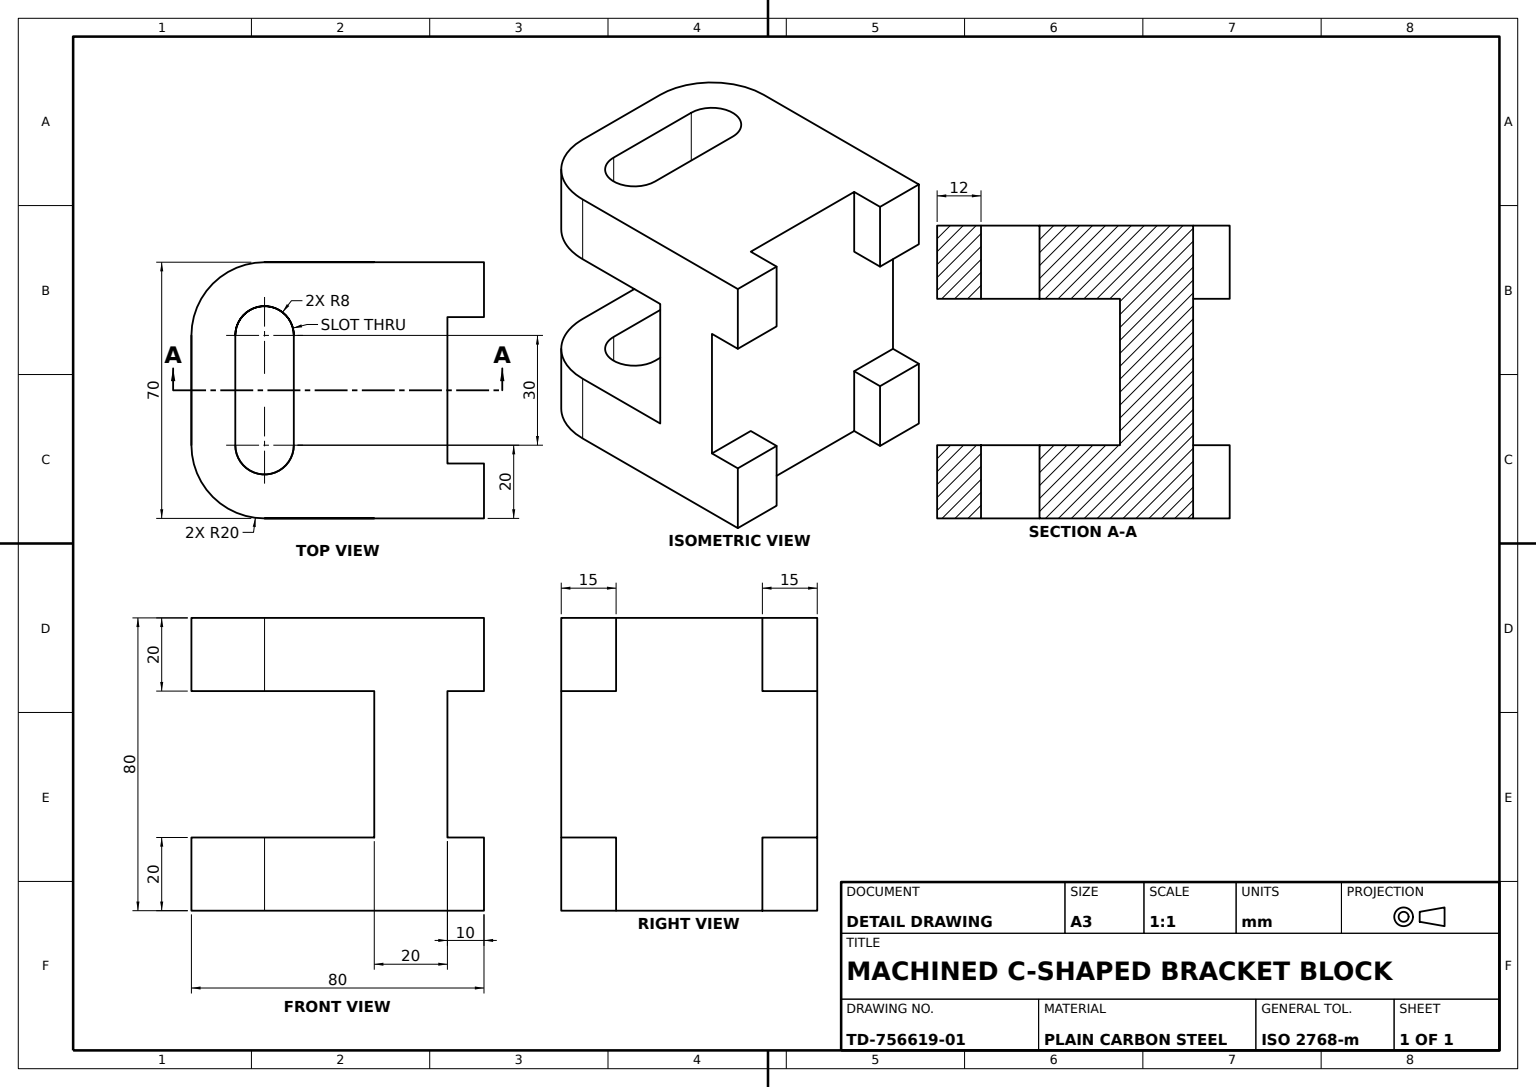
SolidWorks part; units mm, degrees
material "Plain Carbon Steel"
ref_plane "Front Plane" through (0, 0, 0) normal (0, 0, 1) x (1, 0, 0)
ref_plane "Top Plane" through (0, 0, 0) normal (0, 1, 0) x (1, 0, 0)
ref_plane "Right Plane" through (0, 0, 0) normal (1, 0, 0) x (0, 0, -1)
sketch "Base Plate Sketch" plane through (0, 0, 0) normal (0, 0, 1) x (1, 0, 0)
  line L0 (0, 0) -> (70, 0)
  line L1 (70, 0) -> (70, 70)
  line L2 (70, 70) -> (0, 70)
  line L3 (0, 70) -> (0, 0)
  dimension "D1" = 70
  dimension "D2" = 70
  dimension "D3" = 70
extrude "Base Plate 70x70" add sketch "Base Plate Sketch" along normal blind 20
sketch "Web Block Sketch" plane through (0, 0, 0) normal (0, -1, 0) x (1, 0, 0)
  line L0 (0, 0) -> (15, 0)
  line L1 (0, 0) -> (70, 0) construction
  line L2 (15, 0) -> (15, -10)
  line L3 (15, -10) -> (0, -10)
  line L4 (0, -10) -> (0, 0)
  line L5 (70, 0) -> (55, 0)
  line L6 (55, 0) -> (55, -10)
  line L7 (55, -10) -> (70, -10)
  line L8 (70, -10) -> (70, 0)
  line L9 (70, 20) -> (70, 0) construction
  dimension "D1" = 15
  dimension "D2" = 10
extrude "Web Block" add sketch "Web Block Sketch" against normal blind 25
sketch "Side Block A Sketch" plane through (0, 70, 0) normal (0, 1, 0) x (1, 0, 0)
  line L1 (0, 0) -> (15, 0)
  line L2 (0, 0) -> (0, 10)
  line L3 (0, 10) -> (15, 10)
  line L4 (15, 0) -> (15, 10)
extrude "Side Block A" add sketch "Side Block A Sketch" against normal blind 25
sketch "Side Block B Sketch" plane through (0, 70, 0) normal (0, 1, 0) x (1, 0, 0)
  line L0 (70, 0) -> (55, 0)
  line L1 (55, 0) -> (55, 10)
  line L2 (55, 10) -> (70, 10)
  line L3 (70, 10) -> (70, 0)
extrude "Side Block B" add sketch "Side Block B Sketch" against normal blind 25
sketch "Pocket Cut A Sketch" plane through (70, 0, 0) normal (1, 0, 0) x (0, 0, -1)
  line L0 (0, 45) -> (0, 55)
  line L1 (0, 55) -> (10, 55)
  line L2 (10, 45) -> (10, 70) construction
  line L3 (10, 55) -> (10, 45)
  line L4 (10, 45) -> (0, 45)
extrude "Pocket Cut A" cut sketch "Pocket Cut A Sketch" against normal blind 70
sketch "Pocket Cut B Sketch" plane through (70, 0, 0) normal (1, 0, 0) x (0, 0, -1)
  line L0 (10, 25) -> (0, 25)
  line L1 (0, 25) -> (0, 15)
  line L2 (0, 15) -> (10, 15)
  line L3 (10, 25) -> (10, 0) construction
  line L4 (10, 15) -> (10, 25)
extrude "Pocket Cut B" cut sketch "Pocket Cut B Sketch" against normal blind 70
sketch "Flange A Sketch" plane through (0, 0, 0) normal (0, -1, 0) x (1, 0, 0)
  line L0 (0, 20) -> (70, 20)
  line L1 (70, 20) -> (70, -10)
  line L2 (70, -10) -> (55, -10)
  line L3 (55, -10) -> (55, 0)
  line L4 (15, 0) -> (55, 0) construction
  line L5 (55, 0) -> (55, -10) construction
  line L6 (55, 0) -> (15, 0)
  line L7 (15, 0) -> (15, -10)
  line L8 (15, -10) -> (15, 0) construction
  line L9 (15, -10) -> (0, -10)
  line L10 (0, -10) -> (0, 20)
extrude "Flange A 5mm" add sketch "Flange A Sketch" along normal blind 5
sketch "Flange B Sketch" plane through (0, 70, 0) normal (0, 1, 0) x (1, 0, 0)
  line L0 (0, -20) -> (70, -20)
  line L1 (70, -20) -> (70, 10)
  line L2 (70, 10) -> (55, 10)
  line L3 (55, 10) -> (55, 0)
  line L4 (55, 0) -> (15, 0)
  line L5 (15, 0) -> (15, 10)
  line L6 (15, 10) -> (0, 10)
  line L7 (0, 10) -> (0, -20)
extrude "Flange B 5mm" add sketch "Flange B Sketch" along normal blind 5
sketch "Rounded Tab A Sketch" plane through (0, -5, 0) normal (0, -1, 0) x (1, 0, 0)
  line L0 (0, 20) -> (0, 50)
  line L1 (20, 70) -> (50, 70)
  line L2 (70, 50) -> (70, 20)
  line L3 (70, 20) -> (0, 20)
  arc A0 (70, 50) -> (50, 70) centre (50, 50) ccw
  arc A1 (20, 70) -> (0, 50) centre (20, 50) ccw
  dimension "D1" = 20
extrude "Rounded Tab A" add sketch "Rounded Tab A Sketch" against normal blind 20
sketch "Rounded Tab B Sketch" plane through (0, 75, 0) normal (0, 1, 0) x (1, 0, 0)
  line L0 (0, -20) -> (0, -50)
  line L1 (70, -20) -> (70, -50)
  line L2 (20, -70) -> (50, -70)
  line L3 (0, -20) -> (70, -20)
  arc A0 (0, -50) -> (20, -70) centre (20, -50) ccw
  arc A1 (50, -70) -> (70, -50) centre (50, -50) ccw
extrude "Rounded Tab B" add sketch "Rounded Tab B Sketch" against normal blind 20
sketch "Tab Slots Sketch" plane through (0, -5, 0) normal (0, -1, 0) x (1, 0, 0)
  line L0 (0, 50) -> (0, -10) construction
  line L4 (20, 58) -> (50, 58)
  line L5 (20, 42) -> (50, 42)
  arc A0 (20, 58) -> (20, 42) centre (20, 50) ccw
  arc A1 (50, 42) -> (50, 58) centre (50, 50) ccw
  point P0 (12, 50)
  point P1 (58, 50)
  dimension "D1" = 8
  dimension "D2" = 30
  dimension "D3" = 16
  dimension "D4" = 46
  dimension "D5" = 12
  dimension "D6" = 60
extrude "Tab Slots 8x30 Through" cut sketch "Tab Slots Sketch" against normal blind 80
